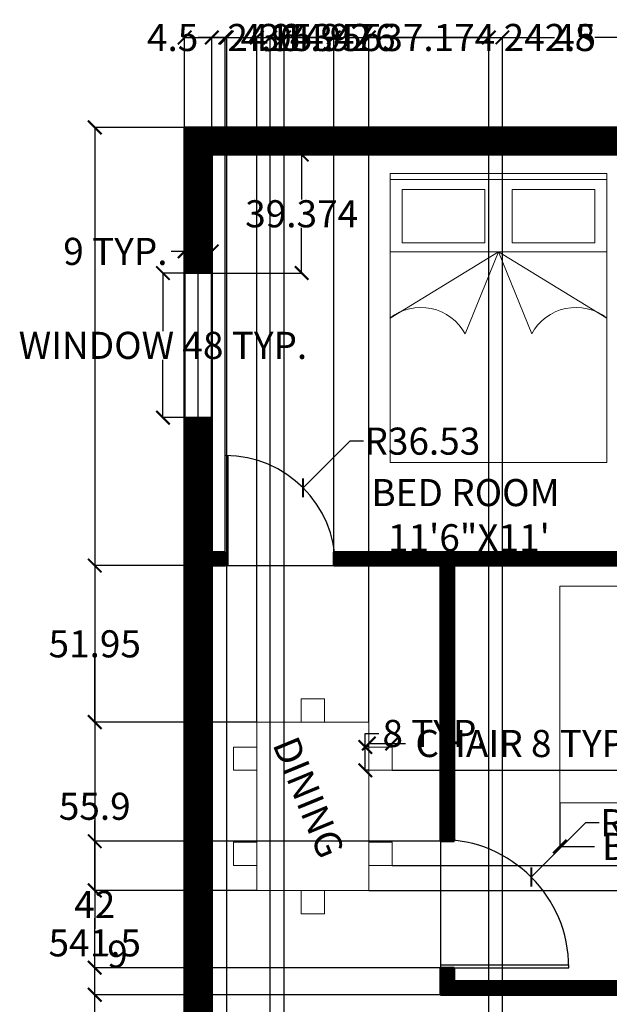
# Model space of a CAD drawing. Units: inches. Extents: x 104 to 466, y -74 to 547.
# Tile 3 of 4: x 104 to 300, y 220 to 547. Entities that reach past the tile are written whole.
import ezdxf

# ---------------------------------------------------------------- set-up
doc = ezdxf.new("R2010")
doc.units = ezdxf.units.IN
doc.header["$MEASUREMENT"] = 0
for name, color, linetype, lineweight in [('A-ANNO-DIMS', 2, 'Continuous', 18), ('A-AREA-IDEN', 7, 'Continuous', 25), ('A-DOOR', 3, 'Continuous', 25), ('A-FURN', 8, 'Continuous', 18), ('A-GLAZ', 4, 'Continuous', 25), ('A-WALL', 7, 'Continuous', 50), ('A-WALL-PATT', 8, 'Continuous', 13)]:
    doc.layers.add(name, color=color, linetype=linetype, lineweight=lineweight)
doc.styles.get("Standard").update_dxf_attribs({"font": 'arial.ttf'})
doc.dimstyles.get("Standard").update_dxf_attribs({"dimtxt": 9, "dimasz": 4.5, "dimexe": 0.18, "dimexo": 0.0625, "dimgap": 0.09, "dimtad": 0, "dimtih": 1, "dimtoh": 1, "dimdec": 1, "dimzin": 0, "dimdsep": 46, "dimlunit": 4, "dimtxsty": 'Standard', "dimblk": 'ARCHTICK', "dimcen": 0.09, "dimadec": 0, "dimazin": 0, "dimtfac": 1, "dimtdec": 1, "dimtofl": 0, "dimtmove": 0, "dimatfit": 3, "dimfxl": 1, "dimtolj": 1, "dimtzin": 0, "dimarcsym": 0})

# ---------------------------------------------------------------- blocks, each defined once
blk = doc.blocks.new('BED-DOUBLE')
for p, q in [((0, 0), (0, 72)), ((0, 72), (96, 72)), ((70, 36), (48, 72)), ((70, 72), (70, 0)), ((94, 72), (94, 0)), ((96, 72), (96, 0)), ((42.75, 47.05), (70, 36)), ((70, 36), (42.75, 24.95)), ((48, 0), (70, 36)), ((96, 0), (0, 0))]:
    blk.add_line(p, q)
for points in [[(90.69, 67.98), (90.69, 40.51), (72.92, 40.51), (72.92, 67.98)], [(90.69, 4.02), (90.69, 31.49), (72.92, 31.49), (72.92, 4.02)]]:
    blk.add_lwpolyline(points, close=True)
for centre, start, end in [((34.78, 61.76), 298.4768, 37.7635), ((34.78, 10.24), 322.2365, 61.5232)]:
    blk.add_arc(centre, 16.73, start, end)
blk = doc.blocks.new('WINDOW-48IN')
for p, q in [((0, 48), (9, 48)), ((0, 0), (0, 48)), ((4.5, 48), (4.5, 0)), ((9, 48), (9, 0)), ((9, 0), (0, 0))]:
    blk.add_line(p, q)
blk = doc.blocks.new('CHAIR-DINING')
blk.add_lwpolyline([(0, 7.73), (7.74, 7.73), (7.74, 0), (0, 0)], close=True)
blk = doc.blocks.new('_ArchTick')
at = {"color": 0, "linetype": 'ByBlock', "const_width": 0.15}
blk.add_lwpolyline([(-0.5, -0.5), (0.5, 0.5)], dxfattribs=at)
blk = doc.blocks.new('*D7')
at = {"layer": 'A-ANNO-DIMS', "color": 0, "lineweight": -2, "transparency": 16777216}
for p, q in [((159.02, 462.67), (151.7, 462.67)), ((151.88, 462.67), (151.88, 443.42)), ((151.88, 414.67), (151.88, 433.92)), ((159.02, 414.67), (151.7, 414.67))]:
    blk.add_line(p, q, dxfattribs=at)
at = {"layer": 'Defpoints', "color": 0, "transparency": 16777216}
for p in [(159.08, 462.67), (151.88, 414.67), (159.08, 414.67)]:
    blk.add_point(p, dxfattribs=at)
at = {"layer": 'A-ANNO-DIMS', "color": 0, "lineweight": -2, "transparency": 16777216, "xscale": 4.5, "yscale": 4.5, "zscale": 4.5}
for p, rotation in [((151.88, 462.67), 90), ((151.88, 414.67), 270)]:
    blk.add_blockref('_ArchTick', p, dxfattribs=dict(at, rotation=rotation))
at = {"layer": 'A-ANNO-DIMS', "color": 0, "transparency": 16777216, "insert": (151.88, 438.67), "char_height": 9, "attachment_point": 5}
blk.add_mtext('\\A1;WINDOW 48 TYP.', dxfattribs=at)
blk = doc.blocks.new('*D8')
at = {"layer": 'A-ANNO-DIMS', "color": 0, "lineweight": -2, "transparency": 16777216}
for p, q in [((159.08, 469.87), (154.58, 469.87)), ((159.08, 462.73), (159.08, 470.05)), ((168.08, 469.87), (159.08, 469.87)), ((168.08, 462.73), (168.08, 470.05))]:
    blk.add_line(p, q, dxfattribs=at)
at = {"layer": 'Defpoints', "color": 0, "transparency": 16777216}
for p in [(159.08, 469.87), (159.08, 462.67), (168.08, 462.67)]:
    blk.add_point(p, dxfattribs=at)
at = {"layer": 'A-ANNO-DIMS', "color": 0, "lineweight": -2, "transparency": 16777216, "xscale": 4.5, "yscale": 4.5, "zscale": 4.5, "rotation": 180}
blk.add_blockref('_ArchTick', (159.08, 469.87), dxfattribs=at)
at = {"layer": 'A-ANNO-DIMS', "color": 0, "lineweight": -2, "transparency": 16777216, "xscale": 4.5, "yscale": 4.5, "zscale": 4.5}
blk.add_blockref('_ArchTick', (168.08, 469.87), dxfattribs=at)
at = {"layer": 'A-ANNO-DIMS', "color": 0, "transparency": 16777216, "insert": (136.09, 469.87), "char_height": 9, "attachment_point": 5}
blk.add_mtext('\\A1;9 TYP.', dxfattribs=at)
blk = doc.blocks.new('*D11')
at = {"layer": 'A-ANNO-DIMS', "color": 0, "lineweight": -2, "transparency": 16777216}
for p, q in [((283.63, 286.66), (283.63, 272.14)), ((379.63, 286.66), (379.63, 272.14)), ((283.63, 272.32), (295.16, 272.32)), ((379.63, 272.32), (368.1, 272.32))]:
    blk.add_line(p, q, dxfattribs=at)
at = {"layer": 'Defpoints', "color": 0, "transparency": 16777216}
for p in [(283.63, 286.72), (379.63, 286.72), (379.63, 272.32)]:
    blk.add_point(p, dxfattribs=at)
at = {"layer": 'A-ANNO-DIMS', "color": 0, "lineweight": -2, "transparency": 16777216, "xscale": 4.5, "yscale": 4.5, "zscale": 4.5, "rotation": 180}
blk.add_blockref('_ArchTick', (283.63, 272.32), dxfattribs=at)
at = {"layer": 'A-ANNO-DIMS', "color": 0, "lineweight": -2, "transparency": 16777216, "xscale": 4.5, "yscale": 4.5, "zscale": 4.5}
blk.add_blockref('_ArchTick', (379.63, 272.32), dxfattribs=at)
at = {"layer": 'A-ANNO-DIMS', "color": 0, "transparency": 16777216, "insert": (331.63, 272.32), "char_height": 9, "attachment_point": 5}
blk.add_mtext('\\A1;BED 96 TYP.', dxfattribs=at)
blk = doc.blocks.new('*D13')
at = {"layer": 'A-ANNO-DIMS', "color": 0, "lineweight": -2, "transparency": 16777216}
for p, q in [((220.21, 305.38), (220.21, 306.66)), ((220.21, 306.48), (227.95, 306.48)), ((227.95, 305.38), (227.95, 306.66)), ((227.95, 306.48), (232.45, 306.48))]:
    blk.add_line(p, q, dxfattribs=at)
at = {"layer": 'Defpoints', "color": 0, "transparency": 16777216}
for p in [(220.21, 305.32), (227.95, 306.48), (227.95, 305.32)]:
    blk.add_point(p, dxfattribs=at)
at = {"layer": 'A-ANNO-DIMS', "color": 0, "lineweight": -2, "transparency": 16777216, "xscale": 4.5, "yscale": 4.5, "zscale": 4.5, "rotation": 180}
blk.add_blockref('_ArchTick', (220.21, 306.48), dxfattribs=at)
at = {"layer": 'A-ANNO-DIMS', "color": 0, "lineweight": -2, "transparency": 16777216, "xscale": 4.5, "yscale": 4.5, "zscale": 4.5}
blk.add_blockref('_ArchTick', (227.95, 306.48), dxfattribs=at)
at = {"layer": 'A-ANNO-DIMS', "color": 0, "transparency": 16777216, "insert": (272.2, 306.48), "char_height": 9, "attachment_point": 5}
blk.add_mtext('\\A1;CHAIR 8 TYP.', dxfattribs=at)
blk = doc.blocks.new('*D14')
at = {"layer": 'A-ANNO-DIMS', "color": 0, "lineweight": -2, "transparency": 16777216}
for p, q in [((219.05, 305.32), (219.05, 309.82)), ((219.05, 309.82), (223.55, 309.82)), ((220.15, 305.32), (218.87, 305.32)), ((219.05, 297.58), (219.05, 305.32)), ((220.15, 297.58), (218.87, 297.58))]:
    blk.add_line(p, q, dxfattribs=at)
at = {"layer": 'Defpoints', "color": 0, "transparency": 16777216}
for p in [(219.05, 305.32), (220.21, 305.32), (220.21, 297.58)]:
    blk.add_point(p, dxfattribs=at)
at = {"layer": 'A-ANNO-DIMS', "color": 0, "lineweight": -2, "transparency": 16777216, "xscale": 4.5, "yscale": 4.5, "zscale": 4.5}
for p, rotation in [((219.05, 305.32), 90), ((219.05, 297.58), 270)]:
    blk.add_blockref('_ArchTick', p, dxfattribs=dict(at, rotation=rotation))
at = {"layer": 'A-ANNO-DIMS', "color": 0, "transparency": 16777216, "insert": (242.06, 309.82), "char_height": 9, "attachment_point": 5}
blk.add_mtext('\\A1;8 TYP.', dxfattribs=at)
blk = doc.blocks.new('*D17')
at = {"layer": 'A-ANNO-DIMS', "color": 0, "lineweight": -2, "transparency": 16777216}
for p, q in [((159.08, 511.11), (159.08, 541.07)), ((159.08, 540.89), (264.95, 540.89)), ((401.58, 540.89), (295.72, 540.89)), ((401.58, 511.11), (401.58, 541.07))]:
    blk.add_line(p, q, dxfattribs=at)
at = {"layer": 'Defpoints', "color": 0, "transparency": 16777216}
for p in [(401.58, 540.89), (159.08, 511.04), (401.58, 511.04)]:
    blk.add_point(p, dxfattribs=at)
at = {"layer": 'A-ANNO-DIMS', "color": 0, "lineweight": -2, "transparency": 16777216, "xscale": 4.5, "yscale": 4.5, "zscale": 4.5, "rotation": 180}
blk.add_blockref('_ArchTick', (159.08, 540.89), dxfattribs=at)
at = {"layer": 'A-ANNO-DIMS', "color": 0, "lineweight": -2, "transparency": 16777216, "xscale": 4.5, "yscale": 4.5, "zscale": 4.5}
blk.add_blockref('_ArchTick', (401.58, 540.89), dxfattribs=at)
at = {"layer": 'A-ANNO-DIMS', "color": 0, "transparency": 16777216, "insert": (280.33, 540.89), "char_height": 9, "attachment_point": 5}
blk.add_mtext('\\A1;242.5', dxfattribs=at)
blk = doc.blocks.new('*D18')
at = {"layer": 'A-ANNO-DIMS', "color": 0, "lineweight": -2, "transparency": 16777216}
for p, q in [((159.02, 511.04), (129.05, 511.04)), ((129.23, 511.04), (129.23, 244.98)), ((129.23, -30.46), (129.23, 235.61)), ((159.02, -30.46), (129.05, -30.46))]:
    blk.add_line(p, q, dxfattribs=at)
at = {"layer": 'Defpoints', "color": 0, "transparency": 16777216}
for p in [(129.23, 511.04), (159.08, 511.04), (159.08, -30.46)]:
    blk.add_point(p, dxfattribs=at)
at = {"layer": 'A-ANNO-DIMS', "color": 0, "lineweight": -2, "transparency": 16777216, "xscale": 4.5, "yscale": 4.5, "zscale": 4.5}
for p, rotation in [((129.23, 511.04), 90), ((129.23, -30.46), 270)]:
    blk.add_blockref('_ArchTick', p, dxfattribs=dict(at, rotation=rotation))
at = {"layer": 'A-ANNO-DIMS', "color": 0, "transparency": 16777216, "insert": (129.23, 240.29), "char_height": 9, "attachment_point": 5}
blk.add_mtext('\\A1;541.5', dxfattribs=at)
blk = doc.blocks.new('*D20')
at = {"layer": 'A-ANNO-DIMS', "color": 0, "lineweight": -2, "transparency": 16777216}
for p, q in [((168.15, 502.04), (198.11, 502.04)), ((197.93, 502.04), (197.93, 487.05)), ((197.93, 462.67), (197.93, 477.67)), ((168.15, 462.67), (198.11, 462.67))]:
    blk.add_line(p, q, dxfattribs=at)
at = {"layer": 'Defpoints', "color": 0, "transparency": 16777216}
for p in [(168.08, 502.04), (168.08, 462.67), (197.93, 462.67)]:
    blk.add_point(p, dxfattribs=at)
at = {"layer": 'A-ANNO-DIMS', "color": 0, "lineweight": -2, "transparency": 16777216, "xscale": 4.5, "yscale": 4.5, "zscale": 4.5}
for p, rotation in [((197.93, 502.04), 90), ((197.93, 462.67), 270)]:
    blk.add_blockref('_ArchTick', p, dxfattribs=dict(at, rotation=rotation))
at = {"layer": 'A-ANNO-DIMS', "color": 0, "transparency": 16777216, "insert": (197.93, 482.36), "char_height": 9, "attachment_point": 5}
blk.add_mtext('\\A1;39.374', dxfattribs=at)
blk = doc.blocks.new('*D26')
at = {"layer": 'A-ANNO-DIMS', "color": 0, "lineweight": -2, "transparency": 16777216}
for p, q in [((168.08, 98.61), (168.08, 541.07)), ((168.08, 540.89), (207.59, 540.89)), ((260.08, 540.89), (220.57, 540.89)), ((260.08, 103.11), (260.08, 541.07))]:
    blk.add_line(p, q, dxfattribs=at)
at = {"layer": 'Defpoints', "color": 0, "transparency": 16777216}
for p in [(260.08, 540.89), (260.08, 103.04), (168.08, 98.54)]:
    blk.add_point(p, dxfattribs=at)
at = {"layer": 'A-ANNO-DIMS', "color": 0, "lineweight": -2, "transparency": 16777216, "xscale": 4.5, "yscale": 4.5, "zscale": 4.5, "rotation": 180}
blk.add_blockref('_ArchTick', (168.08, 540.89), dxfattribs=at)
at = {"layer": 'A-ANNO-DIMS', "color": 0, "lineweight": -2, "transparency": 16777216, "xscale": 4.5, "yscale": 4.5, "zscale": 4.5}
blk.add_blockref('_ArchTick', (260.08, 540.89), dxfattribs=at)
at = {"layer": 'A-ANNO-DIMS', "color": 0, "transparency": 16777216, "insert": (214.08, 540.89), "char_height": 9, "attachment_point": 5}
blk.add_mtext('\\A1;92', dxfattribs=at)
blk = doc.blocks.new('*D31')
at = {"layer": 'A-ANNO-DIMS', "color": 0, "lineweight": -2, "transparency": 16777216}
for p, q in [((168.08, 98.61), (168.08, 541.07)), ((168.08, 540.89), (173.49, 540.89)), ((192.08, 540.89), (186.68, 540.89)), ((192.08, 98.61), (192.08, 541.07))]:
    blk.add_line(p, q, dxfattribs=at)
at = {"layer": 'Defpoints', "color": 0, "transparency": 16777216}
for p in [(192.08, 540.89), (168.08, 98.54), (192.08, 98.54)]:
    blk.add_point(p, dxfattribs=at)
at = {"layer": 'A-ANNO-DIMS', "color": 0, "lineweight": -2, "transparency": 16777216, "xscale": 4.5, "yscale": 4.5, "zscale": 4.5, "rotation": 180}
blk.add_blockref('_ArchTick', (168.08, 540.89), dxfattribs=at)
at = {"layer": 'A-ANNO-DIMS', "color": 0, "lineweight": -2, "transparency": 16777216, "xscale": 4.5, "yscale": 4.5, "zscale": 4.5}
blk.add_blockref('_ArchTick', (192.08, 540.89), dxfattribs=at)
at = {"layer": 'A-ANNO-DIMS', "color": 0, "transparency": 16777216, "insert": (180.08, 540.89), "char_height": 9, "attachment_point": 5}
blk.add_mtext('\\A1;24', dxfattribs=at)
blk = doc.blocks.new('*D37')
at = {"layer": 'A-ANNO-DIMS', "color": 0, "lineweight": -2, "transparency": 16777216}
for p, q in [((264.58, 98.61), (264.58, 541.07)), ((264.58, 540.89), (281.86, 540.89)), ((312.58, 540.89), (295.31, 540.89)), ((312.58, 98.61), (312.58, 541.07))]:
    blk.add_line(p, q, dxfattribs=at)
at = {"layer": 'Defpoints', "color": 0, "transparency": 16777216}
for p in [(312.58, 540.89), (264.58, 98.54), (312.58, 98.54)]:
    blk.add_point(p, dxfattribs=at)
at = {"layer": 'A-ANNO-DIMS', "color": 0, "lineweight": -2, "transparency": 16777216, "xscale": 4.5, "yscale": 4.5, "zscale": 4.5, "rotation": 180}
blk.add_blockref('_ArchTick', (264.58, 540.89), dxfattribs=at)
at = {"layer": 'A-ANNO-DIMS', "color": 0, "lineweight": -2, "transparency": 16777216, "xscale": 4.5, "yscale": 4.5, "zscale": 4.5}
blk.add_blockref('_ArchTick', (312.58, 540.89), dxfattribs=at)
at = {"layer": 'A-ANNO-DIMS', "color": 0, "transparency": 16777216, "insert": (288.58, 540.89), "char_height": 9, "attachment_point": 5}
blk.add_mtext('\\A1;48', dxfattribs=at)
blk = doc.blocks.new('*D39')
at = {"layer": 'A-ANNO-DIMS', "color": 0, "lineweight": -2, "transparency": 16777216}
for p, q in [((183.04, 313.65), (183.04, 541.07)), ((183.04, 540.89), (220.21, 540.89)), ((220.21, 313.65), (220.21, 541.07)), ((220.21, 540.89), (224.71, 540.89))]:
    blk.add_line(p, q, dxfattribs=at)
at = {"layer": 'Defpoints', "color": 0, "transparency": 16777216}
for p in [(220.21, 540.89), (183.04, 313.59), (220.21, 313.59)]:
    blk.add_point(p, dxfattribs=at)
at = {"layer": 'A-ANNO-DIMS', "color": 0, "lineweight": -2, "transparency": 16777216, "xscale": 4.5, "yscale": 4.5, "zscale": 4.5, "rotation": 180}
blk.add_blockref('_ArchTick', (183.04, 540.89), dxfattribs=at)
at = {"layer": 'A-ANNO-DIMS', "color": 0, "lineweight": -2, "transparency": 16777216, "xscale": 4.5, "yscale": 4.5, "zscale": 4.5}
blk.add_blockref('_ArchTick', (220.21, 540.89), dxfattribs=at)
at = {"layer": 'A-ANNO-DIMS', "color": 0, "transparency": 16777216, "insert": (243.46, 540.89), "char_height": 9, "attachment_point": 5}
blk.add_mtext('\\A1;37.174', dxfattribs=at)
blk = doc.blocks.new('*D40')
at = {"layer": 'A-ANNO-DIMS', "color": 0, "lineweight": -2, "transparency": 16777216}
for p, q in [((182.98, 313.59), (129.05, 313.59)), ((129.23, 313.59), (129.23, 290.33)), ((129.23, 257.7), (129.23, 280.96)), ((182.98, 257.7), (129.05, 257.7))]:
    blk.add_line(p, q, dxfattribs=at)
at = {"layer": 'Defpoints', "color": 0, "transparency": 16777216}
for p in [(129.23, 313.59), (183.04, 313.59), (183.04, 257.7)]:
    blk.add_point(p, dxfattribs=at)
at = {"layer": 'A-ANNO-DIMS', "color": 0, "lineweight": -2, "transparency": 16777216, "xscale": 4.5, "yscale": 4.5, "zscale": 4.5}
for p, rotation in [((129.23, 313.59), 90), ((129.23, 257.7), 270)]:
    blk.add_blockref('_ArchTick', p, dxfattribs=dict(at, rotation=rotation))
at = {"layer": 'A-ANNO-DIMS', "color": 0, "transparency": 16777216, "insert": (129.23, 285.64), "char_height": 9, "attachment_point": 5}
blk.add_mtext('\\A1;55.9', dxfattribs=at)
blk = doc.blocks.new('*D41')
at = {"layer": 'A-ANNO-DIMS', "color": 0, "lineweight": -2, "transparency": 16777216}
for p, q in [((228.01, 297.58), (431.61, 297.58)), ((431.43, 297.58), (431.43, 286.47)), ((431.43, 265.97), (431.43, 277.09)), ((228.01, 265.97), (431.61, 265.97))]:
    blk.add_line(p, q, dxfattribs=at)
at = {"layer": 'Defpoints', "color": 0, "transparency": 16777216}
for p in [(227.95, 297.58), (431.43, 297.58), (227.95, 265.97)]:
    blk.add_point(p, dxfattribs=at)
at = {"layer": 'A-ANNO-DIMS', "color": 0, "lineweight": -2, "transparency": 16777216, "xscale": 4.5, "yscale": 4.5, "zscale": 4.5}
for p, rotation in [((431.43, 297.58), 90), ((431.43, 265.97), 270)]:
    blk.add_blockref('_ArchTick', p, dxfattribs=dict(at, rotation=rotation))
at = {"layer": 'A-ANNO-DIMS', "color": 0, "transparency": 16777216, "insert": (431.43, 281.78), "char_height": 9, "attachment_point": 5}
blk.add_mtext('\\A1;31.614', dxfattribs=at)
blk = doc.blocks.new('*D42')
at = {"layer": 'A-ANNO-DIMS', "color": 0, "lineweight": -2, "transparency": 16777216}
for p, q in [((228.01, 265.97), (431.61, 265.97)), ((431.43, 265.97), (431.43, 257.7)), ((220.28, 257.7), (431.61, 257.7)), ((431.43, 257.7), (431.43, 253.19)), ((431.43, 253.19), (426.93, 253.19))]:
    blk.add_line(p, q, dxfattribs=at)
at = {"layer": 'Defpoints', "color": 0, "transparency": 16777216}
for p in [(227.95, 265.97), (220.21, 257.7), (431.43, 257.7)]:
    blk.add_point(p, dxfattribs=at)
at = {"layer": 'A-ANNO-DIMS', "color": 0, "lineweight": -2, "transparency": 16777216, "xscale": 4.5, "yscale": 4.5, "zscale": 4.5}
for p, rotation in [((431.43, 265.97), 90), ((431.43, 257.7), 270)]:
    blk.add_blockref('_ArchTick', p, dxfattribs=dict(at, rotation=rotation))
at = {"layer": 'A-ANNO-DIMS', "color": 0, "transparency": 16777216, "insert": (411.62, 253.19), "char_height": 9, "attachment_point": 5}
blk.add_mtext('\\A1;8.275', dxfattribs=at)
blk = doc.blocks.new('*D43')
at = {"layer": 'A-ANNO-DIMS', "color": 0, "lineweight": -2, "transparency": 16777216}
for p, q in [((172.58, 365.61), (172.58, 541.07)), ((172.58, 540.89), (184.05, 540.89)), ((208.58, 540.89), (197.11, 540.89)), ((208.58, 365.61), (208.58, 541.07))]:
    blk.add_line(p, q, dxfattribs=at)
at = {"layer": 'Defpoints', "color": 0, "transparency": 16777216}
for p in [(172.58, 540.89), (172.58, 365.54), (208.58, 365.54)]:
    blk.add_point(p, dxfattribs=at)
at = {"layer": 'A-ANNO-DIMS', "color": 0, "lineweight": -2, "transparency": 16777216, "xscale": 4.5, "yscale": 4.5, "zscale": 4.5, "rotation": 180}
blk.add_blockref('_ArchTick', (172.58, 540.89), dxfattribs=at)
at = {"layer": 'A-ANNO-DIMS', "color": 0, "lineweight": -2, "transparency": 16777216, "xscale": 4.5, "yscale": 4.5, "zscale": 4.5}
blk.add_blockref('_ArchTick', (208.58, 540.89), dxfattribs=at)
at = {"layer": 'A-ANNO-DIMS', "color": 0, "transparency": 16777216, "insert": (190.58, 540.89), "char_height": 9, "attachment_point": 5}
blk.add_mtext('\\A1;36', dxfattribs=at)
blk = doc.blocks.new('*D44')
at = {"layer": 'A-ANNO-DIMS', "color": 0, "lineweight": -2, "transparency": 16777216}
for p, q in [((168.08, 540.89), (163.58, 540.89)), ((168.08, 365.61), (168.08, 541.07)), ((172.58, 540.89), (168.08, 540.89)), ((172.58, 365.61), (172.58, 541.07))]:
    blk.add_line(p, q, dxfattribs=at)
at = {"layer": 'Defpoints', "color": 0, "transparency": 16777216}
for p in [(168.08, 540.89), (168.08, 365.54), (172.58, 365.54)]:
    blk.add_point(p, dxfattribs=at)
at = {"layer": 'A-ANNO-DIMS', "color": 0, "lineweight": -2, "transparency": 16777216, "xscale": 4.5, "yscale": 4.5, "zscale": 4.5, "rotation": 180}
blk.add_blockref('_ArchTick', (168.08, 540.89), dxfattribs=at)
at = {"layer": 'A-ANNO-DIMS', "color": 0, "lineweight": -2, "transparency": 16777216, "xscale": 4.5, "yscale": 4.5, "zscale": 4.5}
blk.add_blockref('_ArchTick', (172.58, 540.89), dxfattribs=at)
at = {"layer": 'A-ANNO-DIMS', "color": 0, "transparency": 16777216, "insert": (155.09, 540.89), "char_height": 9, "attachment_point": 5}
blk.add_mtext('\\A1;4.5', dxfattribs=at)
blk = doc.blocks.new('*D45')
at = {"layer": 'A-ANNO-DIMS', "color": 0, "lineweight": -2, "transparency": 16777216}
for p, q in [((244.02, 274.04), (129.05, 274.04)), ((129.23, 274.04), (129.23, 257.65)), ((129.23, 232.04), (129.23, 248.44)), ((244.02, 232.04), (129.05, 232.04))]:
    blk.add_line(p, q, dxfattribs=at)
at = {"layer": 'Defpoints', "color": 0, "transparency": 16777216}
for p in [(129.23, 274.04), (244.08, 274.04), (244.08, 232.04)]:
    blk.add_point(p, dxfattribs=at)
at = {"layer": 'A-ANNO-DIMS', "color": 0, "lineweight": -2, "transparency": 16777216, "xscale": 4.5, "yscale": 4.5, "zscale": 4.5}
for p, rotation in [((129.23, 274.04), 90), ((129.23, 232.04), 270)]:
    blk.add_blockref('_ArchTick', p, dxfattribs=dict(at, rotation=rotation))
at = {"layer": 'A-ANNO-DIMS', "color": 0, "transparency": 16777216, "insert": (129.23, 253.04), "char_height": 9, "attachment_point": 5}
blk.add_mtext('\\A1;42', dxfattribs=at)
blk = doc.blocks.new('*D46')
at = {"layer": 'A-ANNO-DIMS', "color": 0, "lineweight": -2, "transparency": 16777216}
for p, q in [((129.23, 232.04), (129.23, 236.54)), ((129.23, 236.54), (133.73, 236.54)), ((244.02, 232.04), (129.05, 232.04)), ((129.23, 223.04), (129.23, 232.04)), ((244.02, 223.04), (129.05, 223.04))]:
    blk.add_line(p, q, dxfattribs=at)
at = {"layer": 'Defpoints', "color": 0, "transparency": 16777216}
for p in [(129.23, 232.04), (244.08, 232.04), (244.08, 223.04)]:
    blk.add_point(p, dxfattribs=at)
at = {"layer": 'A-ANNO-DIMS', "color": 0, "lineweight": -2, "transparency": 16777216, "xscale": 4.5, "yscale": 4.5, "zscale": 4.5}
for p, rotation in [((129.23, 232.04), 90), ((129.23, 223.04), 270)]:
    blk.add_blockref('_ArchTick', p, dxfattribs=dict(at, rotation=rotation))
at = {"layer": 'A-ANNO-DIMS', "color": 0, "transparency": 16777216, "insert": (136.78, 236.54), "char_height": 9, "attachment_point": 5}
blk.add_mtext('\\A1;9', dxfattribs=at)
blk = doc.blocks.new('*D50')
at = {"layer": 'A-ANNO-DIMS', "color": 0, "lineweight": -2, "transparency": 16777216}
for p, q in [((173.04, 64.75), (173.04, 541.07)), ((173.04, 540.89), (187.51, 540.89)), ((187.51, 64.75), (187.51, 541.07)), ((187.51, 540.89), (192.01, 540.89))]:
    blk.add_line(p, q, dxfattribs=at)
at = {"layer": 'Defpoints', "color": 0, "transparency": 16777216}
for p in [(187.51, 540.89), (173.04, 64.69), (187.51, 64.69)]:
    blk.add_point(p, dxfattribs=at)
at = {"layer": 'A-ANNO-DIMS', "color": 0, "lineweight": -2, "transparency": 16777216, "xscale": 4.5, "yscale": 4.5, "zscale": 4.5, "rotation": 180}
blk.add_blockref('_ArchTick', (173.04, 540.89), dxfattribs=at)
at = {"layer": 'A-ANNO-DIMS', "color": 0, "lineweight": -2, "transparency": 16777216, "xscale": 4.5, "yscale": 4.5, "zscale": 4.5}
blk.add_blockref('_ArchTick', (187.51, 540.89), dxfattribs=at)
at = {"layer": 'A-ANNO-DIMS', "color": 0, "transparency": 16777216, "insert": (210.36, 540.89), "char_height": 9, "attachment_point": 5}
blk.add_mtext('\\A1;14.476', dxfattribs=at)
blk = doc.blocks.new('*D53')
at = {"layer": 'A-ANNO-DIMS', "color": 0, "lineweight": -2, "transparency": 16777216}
for p, q in [((168.08, 98.61), (168.08, 541.07)), ((168.08, 540.89), (173.04, 540.89)), ((173.04, 64.75), (173.04, 541.07)), ((173.04, 540.89), (177.54, 540.89))]:
    blk.add_line(p, q, dxfattribs=at)
at = {"layer": 'Defpoints', "color": 0, "transparency": 16777216}
for p in [(173.04, 540.89), (168.08, 98.54), (173.04, 64.69)]:
    blk.add_point(p, dxfattribs=at)
at = {"layer": 'A-ANNO-DIMS', "color": 0, "lineweight": -2, "transparency": 16777216, "xscale": 4.5, "yscale": 4.5, "zscale": 4.5, "rotation": 180}
blk.add_blockref('_ArchTick', (168.08, 540.89), dxfattribs=at)
at = {"layer": 'A-ANNO-DIMS', "color": 0, "lineweight": -2, "transparency": 16777216, "xscale": 4.5, "yscale": 4.5, "zscale": 4.5}
blk.add_blockref('_ArchTick', (173.04, 540.89), dxfattribs=at)
at = {"layer": 'A-ANNO-DIMS', "color": 0, "transparency": 16777216, "insert": (192.99, 540.89), "char_height": 9, "attachment_point": 5}
blk.add_mtext('\\A1;4.953', dxfattribs=at)
blk = doc.blocks.new('*D54')
at = {"layer": 'A-ANNO-DIMS', "color": 0, "lineweight": -2, "transparency": 16777216}
for p, q in [((168.02, 365.54), (129.05, 365.54)), ((129.23, 365.54), (129.23, 344.25)), ((129.23, 313.59), (129.23, 334.88)), ((182.98, 313.59), (129.05, 313.59))]:
    blk.add_line(p, q, dxfattribs=at)
at = {"layer": 'Defpoints', "color": 0, "transparency": 16777216}
for p in [(129.23, 365.54), (168.08, 365.54), (183.04, 313.59)]:
    blk.add_point(p, dxfattribs=at)
at = {"layer": 'A-ANNO-DIMS', "color": 0, "lineweight": -2, "transparency": 16777216, "xscale": 4.5, "yscale": 4.5, "zscale": 4.5}
for p, rotation in [((129.23, 365.54), 90), ((129.23, 313.59), 270)]:
    blk.add_blockref('_ArchTick', p, dxfattribs=dict(at, rotation=rotation))
at = {"layer": 'A-ANNO-DIMS', "color": 0, "transparency": 16777216, "insert": (129.23, 339.57), "char_height": 9, "attachment_point": 5}
blk.add_mtext('\\A1;51.95', dxfattribs=at)
blk = doc.blocks.new('*D55')
at = {"layer": 'A-ANNO-DIMS', "color": 0, "lineweight": -2, "transparency": 16777216}
for p, q in [((168.08, 365.61), (168.08, 541.07)), ((168.08, 540.89), (183.04, 540.89)), ((183.04, 313.65), (183.04, 541.07)), ((183.04, 540.89), (187.54, 540.89))]:
    blk.add_line(p, q, dxfattribs=at)
at = {"layer": 'Defpoints', "color": 0, "transparency": 16777216}
for p in [(183.04, 540.89), (168.08, 365.54), (183.04, 313.59)]:
    blk.add_point(p, dxfattribs=at)
at = {"layer": 'A-ANNO-DIMS', "color": 0, "lineweight": -2, "transparency": 16777216, "xscale": 4.5, "yscale": 4.5, "zscale": 4.5, "rotation": 180}
blk.add_blockref('_ArchTick', (168.08, 540.89), dxfattribs=at)
at = {"layer": 'A-ANNO-DIMS', "color": 0, "lineweight": -2, "transparency": 16777216, "xscale": 4.5, "yscale": 4.5, "zscale": 4.5}
blk.add_blockref('_ArchTick', (183.04, 540.89), dxfattribs=at)
at = {"layer": 'A-ANNO-DIMS', "color": 0, "transparency": 16777216, "insert": (205.92, 540.89), "char_height": 9, "attachment_point": 5}
blk.add_mtext('\\A1;14.955', dxfattribs=at)
blk = doc.blocks.new('*D61')
at = {"layer": 'A-ANNO-DIMS', "color": 0, "lineweight": -2, "transparency": 16777216}
for p, q in [((292.21, 280.18), (274.17, 262.13)), ((296.71, 280.18), (292.21, 280.18)), ((244.08, 231.95), (244.08, 232.13)), ((243.99, 232.04), (244.17, 232.04))]:
    blk.add_line(p, q, dxfattribs=at)
at = {"layer": 'Defpoints', "color": 0, "transparency": 16777216}
for p in [(274.17, 262.13), (244.08, 232.04)]:
    blk.add_point(p, dxfattribs=at)
at = {"layer": 'A-ANNO-DIMS', "color": 0, "lineweight": -2, "transparency": 16777216, "xscale": 4.5, "yscale": 4.5, "zscale": 4.5, "rotation": 225.0001695155098}
blk.add_blockref('_ArchTick', (274.17, 262.13), dxfattribs=at)
at = {"layer": 'A-ANNO-DIMS', "color": 0, "transparency": 16777216, "insert": (316.28, 280.18), "char_height": 9, "attachment_point": 5}
blk.add_mtext('\\A1;R42.54', dxfattribs=at)
blk = doc.blocks.new('*D62')
at = {"layer": 'A-ANNO-DIMS', "color": 0, "lineweight": -2, "transparency": 16777216}
for p, q in [((213.91, 406.87), (198.42, 391.38)), ((218.41, 406.87), (213.91, 406.87)), ((172.49, 365.54), (172.67, 365.54)), ((172.58, 365.45), (172.58, 365.63))]:
    blk.add_line(p, q, dxfattribs=at)
at = {"layer": 'Defpoints', "color": 0, "transparency": 16777216}
for p in [(198.42, 391.38), (172.58, 365.54)]:
    blk.add_point(p, dxfattribs=at)
at = {"layer": 'A-ANNO-DIMS', "color": 0, "lineweight": -2, "transparency": 16777216, "xscale": 4.5, "yscale": 4.5, "zscale": 4.5, "rotation": 224.9990883721471}
blk.add_blockref('_ArchTick', (198.42, 391.38), dxfattribs=at)
at = {"layer": 'A-ANNO-DIMS', "color": 0, "transparency": 16777216, "insert": (238, 406.87), "char_height": 9, "attachment_point": 5}
blk.add_mtext('\\A1;R36.53', dxfattribs=at)

msp = doc.modelspace()

# ---------------------------------------------------------------- hatches: boundary and pattern name
at = {"layer": 'A-WALL-PATT'}
h = msp.add_hatch(dxfattribs=at)
h.set_pattern_fill('ANSI31', color=256)
h.set_pattern_definition([(45, (-366.28003, -301.99136), (-0.088388348, 0.088388348), [])])
h.paths.add_polyline_path([(401.5842, 137.0851), (401.5842, 171.2112), (392.5842, 171.2112), (392.5842, 167.545), (332.0842, 167.545), (332.0842, 137.0851), (332.0842, 103.045), (312.5842, 103.045), (312.5842, 98.545), (392.5842, 98.545), (392.5842, -9.455), (392.5842, -30.455), (401.5842, -30.455), (401.5842, 31.361)])
h.paths.add_polyline_path([(392.5842, 103.045), (336.5842, 103.045), (336.5842, 137.0851), (336.5842, 163.045), (392.5842, 163.045), (392.5842, 137.0851)], flags=16)
h.paths.add_polyline_path([(401.5842, 292.5416), (392.5842, 292.5416), (392.5842, 227.545), (248.5842, 227.545), (248.5842, 232.045), (244.0842, 232.045), (244.0842, 223.045), (248.5842, 223.045), (392.5842, 223.045), (392.5842, 219.2112), (401.5842, 219.2112)])
h.paths.add_polyline_path([(401.5842, 388.2533), (392.5842, 388.2533), (392.5842, 370.045), (340.5842, 370.045), (340.5842, 369.865, -0.03576944), (340.8936, 365.545), (392.5842, 365.545), (392.5842, 340.5416), (401.5842, 340.5416)], flags=17)
h.paths.add_polyline_path([(401.5842, 453.4958), (392.5842, 453.4958), (392.5842, 438.045), (310.5842, 438.045), (310.5842, 467.545), (306.0842, 467.545), (306.0842, 370.045), (208.837, 370.045, -0.03088397), (209.1152, 365.545), (244.0842, 365.545), (244.0842, 274.587, -0.0265002), (248.5842, 274.3483), (248.5842, 365.545), (306.0842, 365.545), (310.5842, 365.545), (310.5842, 370.045), (310.5842, 433.545), (392.5842, 433.545), (392.5842, 424.2533), (401.5842, 424.2533)])
h.paths.add_polyline_path([(168.0842, 365.545), (172.5842, 365.545), (172.5842, 370.045), (168.0842, 370.045), (168.0842, 414.671), (159.0842, 414.671), (159.0842, 214.5244), (168.0842, 214.5244)])
h.paths.add_polyline_path([(168.0842, 98.545), (224.0842, 98.545), (224.0842, 103.045), (168.0842, 103.045), (168.0842, 137.0851), (168.0842, 166.5244), (159.0842, 166.5244), (159.0842, 137.0851), (159.0842, 43.0309), (159.0842, -30.455), (168.0842, -30.455), (177.7316, -30.455), (177.7316, -21.455), (168.0842, -21.455), (168.0842, 35.9487)])
h.paths.add_polyline_path([(264.5842, -21.455), (264.5842, 98.545), (264.5842, 103.045), (260.3643, 103.045, -0.03109877), (260.0842, 98.545), (260.0842, -21.455), (248.5842, -21.455), (213.7316, -21.455), (213.7316, -30.455), (248.5842, -30.455), (264.5842, -30.455)])
h.paths.add_polyline_path([(401.5842, 511.045), (159.0842, 511.045), (159.0842, 462.671), (168.0842, 462.671), (168.0842, 502.045), (306.0842, 502.045), (306.0842, 497.545), (310.5842, 497.545), (310.5842, 502.045), (392.5842, 502.045), (392.5842, 489.4958), (401.5842, 489.4958)])

# ---------------------------------------------------------------- linework, layer by layer
at = {"layer": 'A-DOOR'}
for p, q in [((172.5842, 365.545), (172.5842, 402.076)), ((173.5842, 365.545), (173.5842, 402.0623)), ((172.5842, 365.545), (208.5842, 365.545)), ((244.0842, 274.045), (244.0842, 232.045)), ((244.0842, 233.045), (286.6144, 233.045)), ((244.0842, 232.045), (286.6262, 232.045))]:
    msp.add_line(p, q, dxfattribs=at)
for centre, radius in [((172.5842, 365.545), 36.531), ((244.0842, 232.045), 42.542)]:
    msp.add_arc(centre, radius, 0, 90, dxfattribs=at)
at = {"layer": 'A-FURN'}
for p, q in [((183.0397, 313.5923), (220.2136, 313.5923)), ((183.0397, 257.695), (183.0397, 313.5923)), ((220.2136, 313.5923), (220.2136, 257.695)), ((220.2136, 257.695), (183.0397, 257.695))]:
    msp.add_line(p, q, dxfattribs=at)
at = {"layer": 'A-WALL'}
for p, q in [((159.0842, 511.045), (159.0842, 137.0851)), ((159.0842, 511.045), (401.5842, 511.045)), ((168.0842, 502.045), (168.0842, 370.045)), ((168.0842, 502.045), (306.0842, 502.045)), ((168.0842, 370.045), (172.5842, 370.045)), ((172.5842, 370.045), (172.5842, 365.545)), ((208.5842, 370.045), (208.5842, 365.545)), ((208.5842, 370.045), (306.0842, 370.045)), ((168.0842, 365.545), (172.5842, 365.545)), ((168.0842, 365.545), (168.0842, 137.0851)), ((208.5842, 365.545), (244.0842, 365.545)), ((244.0842, 365.545), (244.0842, 274.045)), ((248.5842, 365.545), (248.5842, 274.045)), ((248.5842, 365.545), (306.0842, 365.545)), ((248.5842, 274.045), (244.0842, 274.045)), ((248.5842, 232.045), (244.0842, 232.045)), ((244.0842, 232.045), (244.0842, 223.045)), ((248.5842, 232.045), (248.5842, 227.545)), ((248.5842, 227.545), (392.5842, 227.545)), ((248.5842, 223.045), (244.0842, 223.045)), ((248.5842, 223.045), (392.5842, 223.045))]:
    msp.add_line(p, q, dxfattribs=at)

# ---------------------------------------------------------------- block references
at = {"layer": 'A-FURN', "rotation": 89.99999999999999}
msp.add_blockref('BED-DOUBLE', (299.2635, 399.7399), dxfattribs=at)
at = {"layer": 'A-FURN'}
for name, p in [('BED-DOUBLE', (283.632, 286.724)), ('CHAIR-DINING', (197.7583, 313.5923)), ('CHAIR-DINING', (175.3027, 297.584)), ('CHAIR-DINING', (220.214, 297.584)), ('CHAIR-DINING', (175.3027, 265.9699)), ('CHAIR-DINING', (220.214, 265.9699)), ('CHAIR-DINING', (197.7583, 249.9616))]:
    msp.add_blockref(name, p, dxfattribs=at)
at = {"layer": 'A-GLAZ', "rotation": 180}
msp.add_blockref('WINDOW-48IN', (168.0843, 462.6712), dxfattribs=at)

# ---------------------------------------------------------------- texts
at = {"layer": 'A-AREA-IDEN', "insert": (221.0861, 394.2863), "char_height": 9, "attachment_point": 1}
msp.add_mtext_dynamic_manual_height_columns('BED ROOM\\P  11\'6"X11\'', width=401.09946, gutter_width=1, heights=[0], dxfattribs=at)
at = {"layer": 'A-AREA-IDEN', "insert": (193.3082, 317.3042), "char_height": 9, "attachment_point": 1, "rotation": 292.335928}
msp.add_mtext_dynamic_manual_height_columns('   DINING', width=401.09946, gutter_width=1, heights=[0], dxfattribs=at)

# ---------------------------------------------------------------- dimensions: what is measured, and where the dimension line sits
at = {"layer": 'A-ANNO-DIMS'}
for base, p1, p2, override, picture, middle in [((168.0842, 540.895), (172.5842, 365.545), (168.0842, 365.545), {"dimdec": 1, "dimlfac": 1, "dimrnd": 0, "dimzin": 0, "dimdsep": 46, "dimlunit": 2}, '*D44', (155.0866, 540.895)), ((401.5842, 540.895), (159.0842, 511.045), (401.5842, 511.045), {"dimdec": 1, "dimlfac": 1, "dimrnd": 0, "dimzin": 0, "dimdsep": 46, "dimlunit": 2}, '*D17', (280.3342, 540.895)), ((260.0842, 540.895), (168.0842, 98.545), (260.0842, 103.045), {"dimdec": 0, "dimlfac": 1, "dimrnd": 0, "dimzin": 0, "dimdsep": 46, "dimlunit": 2}, '*D26', (214.0842, 540.895)), ((192.0842, 540.895), (168.0842, 98.545), (192.0842, 98.545), {"dimdec": 0, "dimlfac": 1, "dimrnd": 0, "dimzin": 0, "dimdsep": 46, "dimlunit": 2}, '*D31', (180.0842, 540.895)), ((173.0369, 540.895), (168.0842, 98.545), (173.0369, 64.6884), {"dimdec": 3, "dimlfac": 1, "dimrnd": 0, "dimzin": 0, "dimdsep": 46, "dimlunit": 2}, '*D53', (192.9932, 540.895)), ((183.03966, 540.89499), (168.08417, 365.54499), (183.03966, 313.59226), {"dimdec": 3, "dimlfac": 1, "dimrnd": 0, "dimzin": 0, "dimdsep": 46, "dimlunit": 2}, '*D55', (205.92127, 540.89499)), ((172.5842, 540.895), (208.5842, 365.545), (172.5842, 365.545), {"dimdec": 0, "dimlfac": 1, "dimrnd": 0, "dimzin": 0, "dimdsep": 46, "dimlunit": 2}, '*D43', (190.5842, 540.895)), ((187.5133, 540.895), (173.0369, 64.6884), (187.5133, 64.6884), {"dimdec": 3, "dimlfac": 1, "dimrnd": 0, "dimzin": 0, "dimdsep": 46, "dimlunit": 2}, '*D50', (210.3581, 540.895)), ((220.2136, 540.895), (183.0397, 313.5923), (220.2136, 313.5923), {"dimdec": 3, "dimlfac": 1, "dimrnd": 0, "dimzin": 0, "dimdsep": 46, "dimlunit": 2}, '*D39', (243.4636, 540.895)), ((312.5842, 540.895), (264.5842, 98.545), (312.5842, 98.545), {"dimdec": 0, "dimlfac": 1, "dimrnd": 0, "dimzin": 0, "dimdsep": 46, "dimlunit": 2}, '*D37', (288.5842, 540.895))]:
    dim = msp.add_linear_dim(base=base, p1=p1, p2=p2, dimstyle='Standard', override=override, dxfattribs=at)
    dim.commit()
    dim.dimension.update_dxf_attribs({"geometry": picture, "text_midpoint": middle})
for base, p1, p2, angle, override, picture, middle in [((129.2342, 511.045), (159.0842, -30.455), (159.0842, 511.045), 90, {"dimdec": 1, "dimlfac": 1, "dimrnd": 0, "dimzin": 0, "dimdsep": 46, "dimlunit": 2}, '*D18', (129.2342, 240.295)), ((197.9342, 462.671), (168.0842, 502.045), (168.0842, 462.671), 270, {"dimdec": 3, "dimlfac": 1, "dimrnd": 0, "dimzin": 0, "dimdsep": 46, "dimlunit": 2}, '*D20', (197.9342, 482.358)), ((129.2342, 365.545), (183.0397, 313.5923), (168.0842, 365.545), 90, {"dimdec": 2, "dimlfac": 1, "dimrnd": 0, "dimzin": 0, "dimdsep": 46, "dimlunit": 2}, '*D54', (129.2342, 339.5686)), ((129.2342, 313.5923), (183.0397, 257.695), (183.0397, 313.5923), 90, {"dimdec": 1, "dimlfac": 1, "dimrnd": 0, "dimzin": 0, "dimdsep": 46, "dimlunit": 2}, '*D40', (129.2342, 285.6436)), ((431.4342, 297.584), (227.951, 265.9698), (227.951, 297.584), 90, {"dimdec": 3, "dimlfac": 1, "dimrnd": 0, "dimzin": 0, "dimdsep": 46, "dimlunit": 2}, '*D41', (431.4342, 281.7769)), ((129.2342, 274.045), (244.0842, 232.045), (244.0842, 274.045), 90, {"dimdec": 0, "dimlfac": 1, "dimrnd": 0, "dimzin": 0, "dimdsep": 46, "dimlunit": 2}, '*D45', (129.2342, 253.045)), ((431.4342, 257.695), (227.951, 265.9698), (220.2136, 257.695), 90, {"dimdec": 3, "dimlfac": 1, "dimrnd": 0, "dimzin": 0, "dimdsep": 46, "dimlunit": 2}, '*D42', (411.6191, 253.195)), ((129.2342, 232.045), (244.0842, 223.045), (244.0842, 232.045), 90, {"dimdec": 0, "dimlfac": 1, "dimrnd": 0, "dimzin": 0, "dimdsep": 46, "dimlunit": 2}, '*D46', (136.7832, 236.545))]:
    dim = msp.add_linear_dim(base=base, p1=p1, p2=p2, angle=angle, dimstyle='Standard', override=override, dxfattribs=at)
    dim.commit()
    dim.dimension.update_dxf_attribs({"geometry": picture, "text_midpoint": middle})
for base, p1, p2, angle, text, picture, middle in [((159.0842, 469.871), (168.0842, 462.671), (159.0842, 462.671), 180, '<> TYP.', '*D8', (136.0859, 469.871)), ((151.8842, 414.671), (159.0842, 462.671), (159.0842, 414.671), 270, 'WINDOW <> TYP.', '*D7', (151.8842, 438.671)), ((219.053, 305.3174), (220.2136, 297.584), (220.2136, 305.3174), 90, '<> TYP.', '*D14', (242.0574, 309.8174))]:
    dim = msp.add_linear_dim(base=base, p1=p1, p2=p2, angle=angle, text=text, dimstyle='Standard', override={"dimdec": 0, "dimlfac": 1, "dimrnd": 0, "dimzin": 0, "dimdsep": 46, "dimlunit": 2}, dxfattribs=at)
    dim.commit()
    dim.dimension.update_dxf_attribs({"geometry": picture, "text_midpoint": middle})
for center, mpoint, picture, middle in [((172.5842, 365.545), (198.4159, 391.3759), '*D62', (237.9968, 406.8745)), ((244.0842, 232.045), (274.1658, 262.1268), '*D61', (316.2782, 280.1759))]:
    dim = msp.add_radius_dim(center=center, mpoint=mpoint, dimstyle='Standard', override={"dimdec": 2, "dimlfac": 1, "dimrnd": 0, "dimzin": 0, "dimdsep": 46, "dimlunit": 2}, dxfattribs=at)
    dim.commit()
    dim.dimension.update_dxf_attribs({"geometry": picture, "text_midpoint": middle, "dimtype": 164})
for base, p1, p2, text, picture, middle in [((227.951, 306.478), (220.2136, 305.3174), (227.951, 305.3174), 'CHAIR <> TYP.', '*D13', (272.203, 306.478)), ((379.632, 272.3239), (283.632, 286.7239), (379.632, 286.7239), 'BED <> TYP.', '*D11', (331.632, 272.3239))]:
    dim = msp.add_linear_dim(base=base, p1=p1, p2=p2, text=text, dimstyle='Standard', override={"dimdec": 0, "dimlfac": 1, "dimrnd": 0, "dimzin": 0, "dimdsep": 46, "dimlunit": 2}, dxfattribs=at)
    dim.commit()
    dim.dimension.update_dxf_attribs({"geometry": picture, "text_midpoint": middle})

doc.saveas('drawing.dxf')
